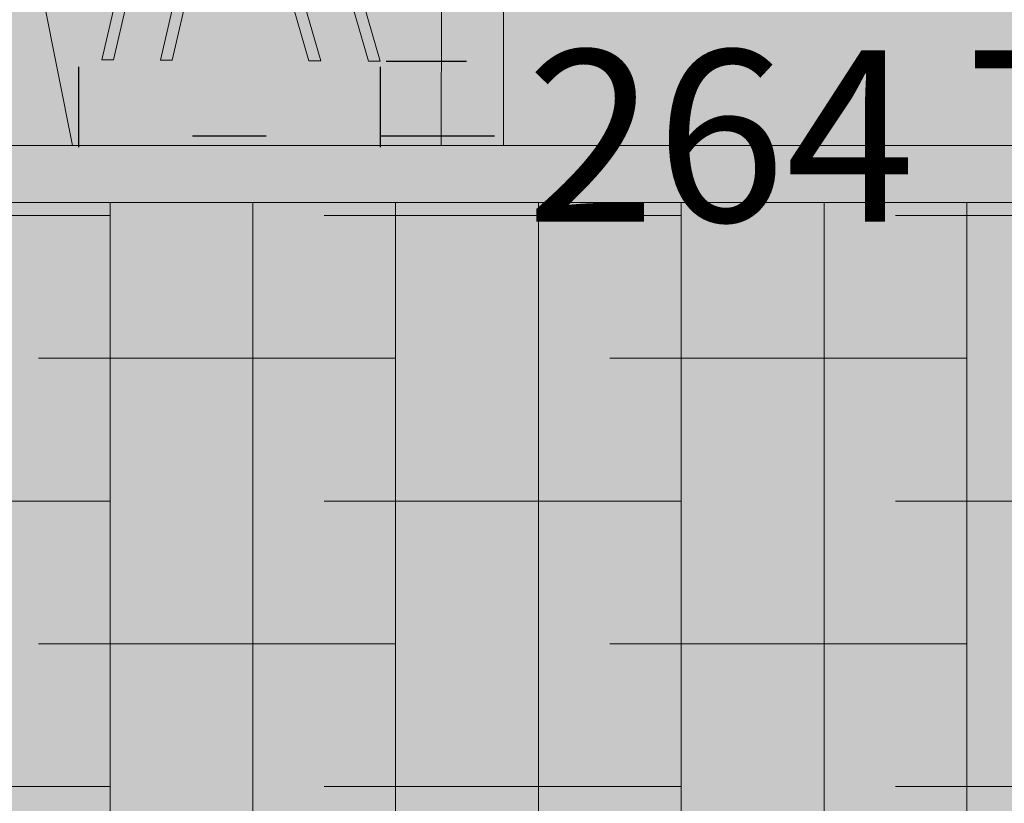
# Model space of a CAD drawing. Units: millimetres. Extents: x 11032 to 26788, y 3406 to 24505.
# Tile 4 of 78: x 15421 to 16283, y 6736 to 7421. Entities that reach past the tile are written whole.
import ezdxf

# ---------------------------------------------------------------- set-up
doc = ezdxf.new("R2010")
doc.units = ezdxf.units.MM
doc.header["$MEASUREMENT"] = 0
for name, color, linetype, lineweight in [('A-ANNO-DIMS', 2, 'Continuous', 18), ('A-FURN', 8, 'Continuous', 13), ('A-FURN-PATT', 8, 'Continuous', 13), ('A-GLAZ', 250, 'Continuous', 20), ('A-WALL-INTR', 8, 'Continuous', 18), ('A-WALL-PLIN-PATT', 253, 'Continuous', 13)]:
    doc.layers.add(name, color=color, linetype=linetype, lineweight=lineweight)
doc.layers.add('A-GLAZ-FRAM-PATT', color=250, linetype='Continuous', lineweight=13, true_color=0x262627)
doc.layers.add('A-WALL-INTR-PATT', color=251, linetype='Continuous', lineweight=13, true_color=0x6c6b6a)
doc.styles.get("Standard").update_dxf_attribs({"font": 'arial.ttf'})
doc.dimstyles.get("Standard").update_dxf_attribs({"dimtxt": 150, "dimasz": 100, "dimexe": 10, "dimexo": 5, "dimgap": 5, "dimtad": 0, "dimtih": 1, "dimtoh": 1, "dimdec": 0, "dimzin": 0, "dimdsep": 46, "dimtxsty": 'Standard', "dimcen": 0.09, "dimadec": 0, "dimazin": 0, "dimtfac": 1, "dimtdec": 0, "dimtofl": 0, "dimtmove": 0, "dimatfit": 3, "dimfxl": 1, "dimtolj": 1, "dimtzin": 0, "dimarcsym": 0})

# ---------------------------------------------------------------- blocks, each defined once
blk = doc.blocks.new('DINING-CHAIR-ELEV')
blk.add_line((228.68, 123.43), (51.04, 132.61))
for points in [[(0, 379.55), (49.45, 435.94), (114.12, 434.53)], [(61.18, 132.09), (30.79, 1.16), (20.53, 1.21), (59.55, 169.26), (0, 379.55), (61.9, 377.89)], [(111.9, 129.47), (82.06, 0.91), (71.8, 0.96), (101.76, 129.99)], [(165.28, 126.71), (201.76, 0.31), (212.19, 0.26), (175.85, 126.16)]]:
    blk.add_lwpolyline(points)
for points in [[(218.11, 123.98), (253.88, 0.05), (264.3, 0), (228.68, 123.43), (238.32, 182.18, 0.148451), (167.47, 178.33), (96.61, 174.48, 0.097012), (61.9, 377.89), (114.12, 434.53, -0.154833), (167.82, 178.46)], [(132.04, 176.4, 0.156877), (88.01, 406.21), (24.72, 407.74)]]:
    blk.add_lwpolyline(points, format="xyb")
blk = doc.blocks.new('*D16')
at = {"layer": 'A-ANNO-DIMS', "color": 0, "lineweight": -2, "transparency": 16777216}
for p, q in [((15741.74, 7821.05), (15812.13, 7821.05)), ((15802.13, 7721.05), (15802.13, 7685.69)), ((15802.13, 7485.11), (15802.13, 7520.47)), ((15741.74, 7385.11), (15812.13, 7385.11))]:
    blk.add_line(p, q, dxfattribs=at)
at = {"layer": 'A-ANNO-DIMS', "color": 0, "transparency": 16777216}
for points in [[(15785.47, 7721.05), (15818.8, 7721.05), (15802.13, 7821.05)], [(15785.47, 7485.11), (15818.8, 7485.11), (15802.13, 7385.11)]]:
    blk.add_solid(points, dxfattribs=at)
at = {"layer": 'Defpoints', "color": 0, "transparency": 16777216}
for p in [(15736.74, 7821.05), (15802.13, 7821.05), (15736.74, 7385.11)]:
    blk.add_point(p, dxfattribs=at)
at = {"layer": 'A-ANNO-DIMS', "color": 0, "transparency": 16777216, "insert": (15802.13, 7603.08), "char_height": 150, "attachment_point": 5}
blk.add_mtext('\\A1;CHAIR 436 TYP.', dxfattribs=at)
blk = doc.blocks.new('*D17')
at = {"layer": 'A-ANNO-DIMS', "color": 0, "lineweight": -2, "transparency": 16777216}
for p, q in [((15472.44, 7380.11), (15472.44, 7309.72)), ((15736.74, 7380.11), (15736.74, 7309.72)), ((15572.44, 7319.72), (15636.74, 7319.72)), ((15736.74, 7319.72), (15836.74, 7319.72))]:
    blk.add_line(p, q, dxfattribs=at)
at = {"layer": 'A-ANNO-DIMS', "color": 0, "transparency": 16777216}
for points in [[(15572.44, 7336.38), (15572.44, 7303.05), (15472.44, 7319.72)], [(15636.74, 7336.38), (15636.74, 7303.05), (15736.74, 7319.72)]]:
    blk.add_solid(points, dxfattribs=at)
at = {"layer": 'Defpoints', "color": 0, "transparency": 16777216}
for p in [(15472.44, 7385.11), (15736.74, 7385.11), (15736.74, 7319.72)]:
    blk.add_point(p, dxfattribs=at)
at = {"layer": 'A-ANNO-DIMS', "color": 0, "transparency": 16777216, "insert": (16266.37, 7319.72), "char_height": 150, "attachment_point": 5}
blk.add_mtext('\\A1;264 TYP.', dxfattribs=at)
blk = doc.blocks.new('*D36')
at = {"layer": 'A-ANNO-DIMS', "color": 0, "lineweight": -2, "transparency": 16777216}
for p, q in [((12301.26, 17115.89), (12301.26, 24416.86)), ((25397.4, 4466.4), (25397.4, 24416.86)), ((12401.26, 24406.86), (18569.2, 24406.86)), ((25297.4, 24406.86), (19129.47, 24406.86))]:
    blk.add_line(p, q, dxfattribs=at)
at = {"layer": 'A-ANNO-DIMS', "color": 0, "transparency": 16777216}
for points in [[(12401.26, 24423.52), (12401.26, 24390.19), (12301.26, 24406.86)], [(25297.4, 24423.52), (25297.4, 24390.19), (25397.4, 24406.86)]]:
    blk.add_solid(points, dxfattribs=at)
at = {"layer": 'Defpoints', "color": 0, "transparency": 16777216}
for p in [(25397.4, 24406.86), (12301.26, 17110.89), (25397.4, 4461.4)]:
    blk.add_point(p, dxfattribs=at)
at = {"layer": 'A-ANNO-DIMS', "color": 0, "transparency": 16777216, "insert": (18849.33, 24406.86), "char_height": 150, "attachment_point": 5}
blk.add_mtext('\\A1;13096', dxfattribs=at)
blk = doc.blocks.new('*D37')
at = {"layer": 'A-ANNO-DIMS', "color": 0, "lineweight": -2, "transparency": 16777216}
for p, q in [((18087.74, 23450.36), (11334.76, 23450.36)), ((11344.76, 23350.36), (11344.76, 14037.46)), ((11344.76, 4561.4), (11344.76, 13874.29)), ((12927.66, 4461.4), (11334.76, 4461.4))]:
    blk.add_line(p, q, dxfattribs=at)
at = {"layer": 'A-ANNO-DIMS', "color": 0, "transparency": 16777216}
for points in [[(11328.1, 23350.36), (11361.43, 23350.36), (11344.76, 23450.36)], [(11328.1, 4561.4), (11361.43, 4561.4), (11344.76, 4461.4)]]:
    blk.add_solid(points, dxfattribs=at)
at = {"layer": 'Defpoints', "color": 0, "transparency": 16777216}
for p in [(11344.76, 23450.36), (18092.74, 23450.36), (12932.66, 4461.4)]:
    blk.add_point(p, dxfattribs=at)
at = {"layer": 'A-ANNO-DIMS', "color": 0, "transparency": 16777216, "insert": (11344.76, 13955.88), "char_height": 150, "attachment_point": 5}
blk.add_mtext('\\A1;18989', dxfattribs=at)
blk = doc.blocks.new('*D49')
at = {"layer": 'A-ANNO-DIMS', "color": 0, "lineweight": -2, "transparency": 16777216}
for p, q in [((17953.45, 10206.41), (17953.45, 3494.9)), ((14996.4, 6406.4), (14996.4, 3494.9)), ((15096.4, 3504.9), (16244.67, 3504.9)), ((17853.45, 3504.9), (16705.18, 3504.9))]:
    blk.add_line(p, q, dxfattribs=at)
at = {"layer": 'A-ANNO-DIMS', "color": 0, "transparency": 16777216}
for points in [[(15096.4, 3521.57), (15096.4, 3488.23), (14996.4, 3504.9)], [(17853.45, 3521.57), (17853.45, 3488.23), (17953.45, 3504.9)]]:
    blk.add_solid(points, dxfattribs=at)
at = {"layer": 'Defpoints', "color": 0, "transparency": 16777216}
for p in [(17953.45, 10211.41), (14996.4, 6411.4), (17953.45, 3504.9)]:
    blk.add_point(p, dxfattribs=at)
at = {"layer": 'A-ANNO-DIMS', "color": 0, "transparency": 16777216, "insert": (16474.93, 3504.9), "char_height": 150, "attachment_point": 5}
blk.add_mtext('\\A1;2957', dxfattribs=at)
blk = doc.blocks.new('*D57')
at = {"layer": 'A-ANNO-DIMS', "color": 0, "lineweight": -2, "transparency": 16777216}
for p, q in [((14994.7, 7266.4), (14994.7, 24416.86)), ((20894.7, 7266.4), (20894.7, 24416.86)), ((15094.7, 24406.86), (17715.98, 24406.86)), ((20794.7, 24406.86), (18173.42, 24406.86))]:
    blk.add_line(p, q, dxfattribs=at)
at = {"layer": 'A-ANNO-DIMS', "color": 0, "transparency": 16777216}
for points in [[(15094.7, 24423.52), (15094.7, 24390.19), (14994.7, 24406.86)], [(20794.7, 24423.52), (20794.7, 24390.19), (20894.7, 24406.86)]]:
    blk.add_solid(points, dxfattribs=at)
at = {"layer": 'Defpoints', "color": 0, "transparency": 16777216}
for p in [(20894.7, 24406.86), (14994.7, 7261.4), (20894.7, 7261.4)]:
    blk.add_point(p, dxfattribs=at)
at = {"layer": 'A-ANNO-DIMS', "color": 0, "transparency": 16777216, "insert": (17944.7, 24406.86), "char_height": 150, "attachment_point": 5}
blk.add_mtext('\\A1;5900', dxfattribs=at)
blk = doc.blocks.new('*D60')
at = {"layer": 'A-ANNO-DIMS', "color": 0, "lineweight": -2, "transparency": 16777216}
for p, q in [((14994.7, 7266.4), (14994.7, 24416.86)), ((16344.7, 7266.4), (16344.7, 24416.86)), ((15094.7, 24406.86), (15448.04, 24406.86)), ((16244.7, 24406.86), (15891.36, 24406.86))]:
    blk.add_line(p, q, dxfattribs=at)
at = {"layer": 'A-ANNO-DIMS', "color": 0, "transparency": 16777216}
for points in [[(15094.7, 24423.52), (15094.7, 24390.19), (14994.7, 24406.86)], [(16244.7, 24423.52), (16244.7, 24390.19), (16344.7, 24406.86)]]:
    blk.add_solid(points, dxfattribs=at)
at = {"layer": 'Defpoints', "color": 0, "transparency": 16777216}
for p in [(16344.7, 24406.86), (14994.7, 7261.4), (16344.7, 7261.4)]:
    blk.add_point(p, dxfattribs=at)
at = {"layer": 'A-ANNO-DIMS', "color": 0, "transparency": 16777216, "insert": (15669.7, 24406.86), "char_height": 150, "attachment_point": 5}
blk.add_mtext('\\A1;1350', dxfattribs=at)
blk = doc.blocks.new('*D69')
at = {"layer": 'A-ANNO-DIMS', "color": 0, "lineweight": -2, "transparency": 16777216}
for p, q in [((13956.97, 9937.95), (14056.97, 9937.95)), ((14056.97, 9937.95), (15432.5, 8990.95)), ((17944.61, 7261.4), (17944.79, 7261.4)), ((17944.7, 7261.31), (17944.7, 7261.49))]:
    blk.add_line(p, q, dxfattribs=at)
at = {"layer": 'A-ANNO-DIMS', "color": 0, "transparency": 16777216}
blk.add_solid([(15441.95, 9004.68), (15423.05, 8977.22), (15514.87, 8934.24)], dxfattribs=at)
at = {"layer": 'Defpoints', "color": 0, "transparency": 16777216}
for p in [(15514.87, 8934.24), (17944.7, 7261.4)]:
    blk.add_point(p, dxfattribs=at)
at = {"layer": 'A-ANNO-DIMS', "color": 0, "transparency": 16777216, "insert": (13494.04, 9937.95), "char_height": 150, "attachment_point": 5}
blk.add_mtext('\\A1;2X R2950', dxfattribs=at)

msp = doc.modelspace()

# ---------------------------------------------------------------- hatches: boundary and pattern name
at = {"layer": 'A-FURN-PATT'}
h = msp.add_hatch(color=256, dxfattribs=at)
h.set_gradient(color1=(153, 27, 30), color2=(153, 38, 0), name='SPHERICAL')
h.paths.add_polyline_path([(15534.344, 7763), (15472.44, 7764.657), (15531.986, 7554.365), (15523.479, 7517.719), (15640.736, 7511.661), (15653.713, 7567.556, 0.0295203), (15639.906, 7563.436), (15569.055, 7559.583, 0.0970121)], flags=16)
h.paths.add_polyline_path([(15560.453, 7791.32), (15534.344, 7763, -0.0970121), (15569.055, 7559.583), (15604.48, 7561.509, 0.1568775)], flags=16)
h.paths.add_polyline_path([(15586.562, 7819.64), (15560.453, 7791.32, -0.1568775), (15604.48, 7561.509), (15640.246, 7563.454, 0.154898)], flags=17)
h.paths.add_polyline_path([(15560.453, 7791.32), (15497.165, 7792.851), (15472.44, 7764.657), (15534.344, 7763)], flags=16)
h.paths.add_polyline_path([(15586.562, 7819.64), (15521.889, 7821.046), (15497.165, 7792.851), (15560.453, 7791.32)], flags=17)
h.paths.add_polyline_path([(15790.874, 7662.689, 0.021469), (15780.879, 7659.53), (15710.028, 7655.677, 0.0970121), (15675.317, 7859.094), (15665.772, 7859.35), (15665.799, 7675.745), (15672.959, 7650.459), (15665.807, 7619.654), (15665.808, 7613.744), (15790.755, 7607.288)], flags=17)
h.paths.add_polyline_path([(15665.772, 7859.35), (15613.413, 7860.751), (15665.799, 7675.745)], flags=16)
h.paths.add_polyline_path([(15701.426, 7887.414), (15665.767, 7888.277), (15665.772, 7859.35), (15675.317, 7859.094)], flags=16)
h.paths.add_polyline_path([(15727.534, 7915.735), (15665.763, 7917.077), (15665.767, 7888.277), (15701.426, 7887.414)], flags=17)
h.paths.add_polyline_path([(15665.763, 7917.077), (15662.862, 7917.14), (15638.137, 7888.946), (15665.767, 7888.277)], flags=17)
h.paths.add_polyline_path([(15665.767, 7888.277), (15638.137, 7888.946), (15613.413, 7860.751), (15665.772, 7859.35)], flags=16)
h.paths.add_polyline_path([(15701.426, 7887.414), (15675.317, 7859.094, -0.0970121), (15710.028, 7655.677), (15745.453, 7657.604, 0.1568775)], flags=16)
h.paths.add_polyline_path([(15844.495, 7664.925), (15844.384, 7864.461), (15821.312, 7945.94), (15870.762, 8002.329), (15935.434, 8000.923, -0.1195917), (15991.005, 7804.617), (16002.667, 7804.617), (16022.264, 7889.032), (15962.718, 8099.323), (16024.622, 8097.666), (16076.839, 8154.307, -0.1548334), (16130.535, 7898.229, -0.1476694), (16201.035, 7901.954), (16191.395, 7843.208), (16202.533, 7804.617), (16299.12, 7804.617), (16297.929, 7808.825), (16347.378, 7865.214), (16412.05, 7863.808, -0.0295496), (16434.494, 7817.915), (16458.237, 7920.19), (16398.691, 8130.481), (16460.595, 8128.825), (16512.813, 8185.465, -0.1548334), (16566.508, 7929.387, -0.1476694), (16637.008, 7933.112), (16627.369, 7874.366), (16647.499, 7804.617), (16830.506, 7804.617), (16830.506, 7793.515), (16650.704, 7793.515), (16662.994, 7750.932), (16652.571, 7750.983), (16640.296, 7793.515), (16490.425, 7793.515), (16480.749, 7751.837), (16470.495, 7751.888), (16480.159, 7793.515), (16443.833, 7793.515, -0.1094051), (16465.746, 7607.731, -0.1476694), (16536.246, 7611.456), (16526.606, 7552.71), (16562.232, 7429.275), (16551.809, 7429.327), (16516.041, 7553.255), (16473.778, 7555.439), (16510.116, 7429.534), (16499.693, 7429.586), (16463.212, 7555.985), (16409.833, 7558.743), (16379.987, 7430.181), (16369.733, 7430.232), (16394.704, 7537.793), (16394.704, 7559.524), (16359.112, 7561.363), (16328.717, 7430.435), (16318.463, 7430.486), (16344.704, 7543.521), (16344.704, 7643.635), (16302.264, 7793.515), (16205.738, 7793.515), (16227.021, 7719.773), (16216.598, 7719.825), (16195.329, 7793.515), (16153.697, 7793.515), (16174.905, 7720.032), (16164.482, 7720.084), (16143.289, 7793.515), (16061.685, 7793.515), (16051.641, 7750.248, -0.0167144), (16059.629, 7748.571), (16049.99, 7689.825), (16085.615, 7566.39), (16075.192, 7566.442), (16039.424, 7690.371), (15997.161, 7692.554), (16033.5, 7566.649), (16023.077, 7566.701), (15986.595, 7693.1), (15933.216, 7695.858), (15903.371, 7567.296), (15893.116, 7567.347), (15923.072, 7696.382), (15882.495, 7698.478), (15852.409, 7568.882), (15877.716, 7481.201), (15867.293, 7481.253), (15842.372, 7567.599), (15841.846, 7567.602), (15842.08, 7568.609), (15831.524, 7605.182), (15790.755, 7607.288), (15790.744, 7602.228), (15825.6, 7481.46), (15815.177, 7481.512), (15778.696, 7607.911), (15725.317, 7610.669), (15701.389, 7507.6), (15736.743, 7385.107), (15726.32, 7385.159), (15696.749, 7487.614), (15695.471, 7482.107), (15685.217, 7482.158), (15691.06, 7507.327), (15690.552, 7509.088), (15650.881, 7511.137), (15649.743, 7506.234), (15684.627, 7385.366), (15674.204, 7385.418), (15645.103, 7486.248), (15644.2, 7482.362), (15633.946, 7482.413), (15639.413, 7505.961), (15637.723, 7511.817), (15584.344, 7514.575), (15554.498, 7386.013), (15544.244, 7386.064), (15574.2, 7515.099), (15533.623, 7517.195), (15503.228, 7386.268), (15492.974, 7386.319), (15531.986, 7554.365), (15472.44, 7764.657), (15497.165, 7792.851), (15521.889, 7821.046), (15586.562, 7819.64, -0.1548334), (15640.257, 7563.563, -0.0287549), (15653.713, 7567.556), (15665.807, 7619.654), (15665.799, 7675.745), (15613.413, 7860.751), (15638.137, 7888.946), (15662.862, 7917.14), (15665.763, 7917.077), (15727.534, 7915.735, -0.1548334), (15781.23, 7659.657, -0.1322263)])
h = msp.add_hatch(color=256, dxfattribs=at)
h.set_gradient(color1=(153, 27, 30), color2=(153, 38, 0), name='SPHERICAL')
h.paths.add_polyline_path([(15710.028, 7655.677), (15745.453, 7657.604, 0.1568775), (15701.426, 7887.414), (15675.317, 7859.094, -0.0970121)], flags=16)
h.paths.add_polyline_path([(15790.755, 7607.288), (15790.874, 7662.689, 0.021469), (15780.879, 7659.53), (15710.028, 7655.677, 0.0970121), (15675.317, 7859.094), (15665.772, 7859.35), (15665.799, 7675.745), (15672.959, 7650.459), (15665.807, 7619.654), (15665.808, 7613.744)], flags=17)
h.paths.add_polyline_path([(15653.713, 7567.556), (15665.807, 7619.654), (15665.799, 7675.745), (15613.413, 7860.751), (15662.862, 7917.14), (15727.534, 7915.735, -0.1548334), (15781.23, 7659.657, -0.1322263), (15844.495, 7664.925), (15844.384, 7864.461), (15821.312, 7945.94), (15883.216, 7944.283), (15935.434, 8000.923, -0.1195917), (15991.005, 7804.617), (16002.667, 7804.617), (16022.264, 7889.032), (15962.718, 8099.323), (16024.622, 8097.666), (16076.839, 8154.307, -0.1548334), (16130.535, 7898.229, -0.1476694), (16201.035, 7901.954), (16191.395, 7843.208), (16202.533, 7804.617), (16830.506, 7804.617), (16830.506, 7793.515), (16205.738, 7793.515), (16227.021, 7719.773), (16216.598, 7719.825), (16195.329, 7793.515), (16153.697, 7793.515), (16174.905, 7720.032), (16164.482, 7720.084), (16143.289, 7793.515), (16061.685, 7793.515), (16051.641, 7750.248, -0.0167144), (16059.629, 7748.571), (16049.99, 7689.825), (16085.615, 7566.39), (16075.192, 7566.442), (16039.424, 7690.371), (15997.161, 7692.554), (16033.5, 7566.649), (16023.077, 7566.701), (15986.595, 7693.1), (15933.216, 7695.858), (15903.371, 7567.296), (15893.116, 7567.347), (15923.072, 7696.382), (15882.495, 7698.478), (15852.409, 7568.882), (15877.716, 7481.201), (15867.293, 7481.253), (15842.372, 7567.599), (15841.846, 7567.602), (15842.08, 7568.609), (15831.524, 7605.182), (15790.755, 7607.288), (15790.744, 7602.228), (15825.6, 7481.46), (15815.177, 7481.512), (15778.696, 7607.911), (15725.317, 7610.669), (15701.389, 7507.6), (15736.743, 7385.107), (15726.32, 7385.159), (15696.749, 7487.614), (15695.471, 7482.107), (15685.217, 7482.158), (15705.262, 7568.502, 0.0841685), (15664.448, 7569.579), (15644.2, 7482.362), (15633.946, 7482.413), (15653.713, 7567.556, 0.0295203), (15639.906, 7563.436), (15569.055, 7559.583, 0.0970121), (15534.344, 7763), (15472.44, 7764.657), (15521.889, 7821.046), (15586.562, 7819.64, -0.1548334), (15640.257, 7563.563, -0.0287549)])
at = {"layer": 'A-GLAZ-FRAM-PATT'}
h = msp.add_hatch(color=256, dxfattribs=at)
h.paths.add_polyline_path([(17944.704, 7311.399), (16344.704, 7311.399), (16344.704, 7261.399), (17944.704, 7261.399)], flags=17)
h.paths.add_polyline_path([(16344.704, 7311.399), (15045.135, 7311.399, -0.9829047), (20844.273, 7311.399), (19544.704, 7311.399), (19544.704, 7261.399), (20894.704, 7261.399, 0.5148441), (16985.951, 10051.255, 0.3202679), (14994.704, 7261.399), (16344.704, 7261.399)])
h.paths.add_polyline_path([(18744.704, 7311.399), (17944.704, 7311.399), (17944.704, 7261.399), (18744.704, 7261.399)], flags=17)
h.paths.add_polyline_path([(19544.704, 7311.399), (18744.704, 7311.399), (18744.704, 7261.399), (19544.704, 7261.399)], flags=17)
h.paths.add_polyline_path([(18694.704, 7361.399), (17994.704, 7361.399), (17994.704, 7311.399), (18694.704, 7311.399)], flags=17)
h.paths.add_polyline_path([(18744.704, 7361.399), (18694.704, 7361.399), (18694.704, 7311.399), (18744.704, 7311.399)], flags=17)
h.paths.add_polyline_path([(17194.704, 7361.399), (17144.704, 7361.399), (17144.704, 7311.399), (17194.704, 7311.399)], flags=17)
h.paths.add_polyline_path([(17431.432, 7361.399), (17194.704, 7361.399), (17194.704, 7311.399), (17431.699, 7311.399)], flags=17)
h.paths.add_polyline_path([(17894.704, 7361.399), (17431.432, 7361.399), (17431.699, 7311.399), (17894.704, 7311.399)], flags=17)
h.paths.add_polyline_path([(17944.704, 7361.399), (17894.704, 7361.399), (17894.704, 7311.399), (17944.704, 7311.399)], flags=17)
h.paths.add_polyline_path([(17994.704, 7361.399), (17944.704, 7361.399), (17944.704, 7311.399), (17994.704, 7311.399)], flags=17)
at = {"layer": 'A-WALL-INTR-PATT'}
msp.add_hatch(color=256, dxfattribs=at).paths.add_polyline_path([(15447.906, 8736.527, 0.0271717), (15302.659, 8457.059), (15381.661, 7740.545), (15467.334, 7311.399), (15790.119, 7311.399), (15790.667, 7566.433), (15778.696, 7607.911), (15725.317, 7610.669), (15701.389, 7507.6), (15736.743, 7385.107), (15726.32, 7385.159), (15696.749, 7487.614), (15695.471, 7482.107), (15685.217, 7482.158), (15691.06, 7507.327), (15690.552, 7509.088), (15650.881, 7511.137), (15649.743, 7506.234), (15684.627, 7385.366), (15674.204, 7385.418), (15645.103, 7486.248), (15644.2, 7482.362), (15633.946, 7482.413), (15639.413, 7505.961), (15637.723, 7511.817), (15584.344, 7514.575), (15554.498, 7386.013), (15544.244, 7386.064), (15574.2, 7515.099), (15533.623, 7517.195), (15503.228, 7386.268), (15492.974, 7386.319), (15531.986, 7554.365), (15472.44, 7764.657)])
h = msp.add_hatch(color=256, dxfattribs=at)
h.paths.add_polyline_path([(15302.659, 8457.059, 0.0281002), (15185.248, 8153.253), (15233.282, 7717.599), (15314.374, 7311.399), (15467.334, 7311.399), (15381.661, 7740.545)])
h.paths.add_polyline_path([(16344.704, 7543.521), (16344.704, 7643.635), (16302.264, 7793.515), (16205.738, 7793.515), (16227.021, 7719.773), (16216.598, 7719.825), (16195.329, 7793.515), (16153.697, 7793.515), (16174.905, 7720.032), (16164.482, 7720.084), (16143.289, 7793.515), (16061.685, 7793.515), (16051.641, 7750.248, -0.0167144), (16059.629, 7748.571), (16049.99, 7689.825), (16085.615, 7566.39), (16075.192, 7566.442), (16039.424, 7690.371), (15997.161, 7692.554), (16033.5, 7566.649), (16023.077, 7566.701), (15986.595, 7693.1), (15933.216, 7695.858), (15903.371, 7567.296), (15893.116, 7567.347), (15923.072, 7696.382), (15882.495, 7698.478), (15852.409, 7568.882), (15877.716, 7481.201), (15867.293, 7481.253), (15844.553, 7560.041), (15844.691, 7311.399), (16344.704, 7311.399), (16344.704, 7499.3), (16328.717, 7430.435), (16318.463, 7430.486)])
h.paths.add_polyline_path([(16742.983, 7793.515), (16650.704, 7793.515), (16662.994, 7750.932), (16652.571, 7750.983), (16640.296, 7793.515), (16598.663, 7793.515), (16610.879, 7751.191), (16600.455, 7751.242), (16588.255, 7793.515), (16490.425, 7793.515), (16480.749, 7751.837), (16470.495, 7751.888), (16480.159, 7793.515), (16443.833, 7793.515, -0.1094051), (16465.746, 7607.731, -0.1476694), (16536.246, 7611.456), (16526.606, 7552.71), (16562.232, 7429.275), (16551.809, 7429.327), (16516.041, 7553.255), (16473.778, 7555.439), (16510.116, 7429.534), (16499.693, 7429.586), (16463.212, 7555.985), (16409.833, 7558.743), (16394.704, 7493.572), (16394.704, 7361.399), (16744.704, 7361.399)])
h.paths.add_polyline_path([(17094.704, 8239.696), (16741.207, 8239.696), (16742.939, 7804.617), (16768.057, 7804.617), (16785.352, 7864.542), (16775.713, 7923.288, -0.1476694), (16846.212, 7919.563, -0.1548334), (16899.908, 8175.64), (16964.58, 8177.046), (17014.03, 8120.657), (16954.484, 7910.365), (16972.017, 7834.84), (16977.75, 7834.965), (17027.199, 7778.576), (16967.653, 7568.284), (17006.665, 7400.238), (16996.411, 7400.187), (16966.016, 7531.114), (16925.439, 7529.018), (16955.395, 7399.983), (16945.141, 7399.932), (16915.295, 7528.494), (16861.916, 7525.736), (16825.435, 7399.337), (16815.012, 7399.285), (16851.35, 7525.19), (16809.087, 7523.007), (16773.319, 7399.078), (16762.896, 7399.026), (16798.521, 7522.461), (16788.882, 7581.207, -0.1476694), (16859.382, 7577.482, -0.1528132), (16911.41, 7830.579), (16902.125, 7870.575), (16848.746, 7867.817), (16830.506, 7804.617), (16830.506, 7793.515), (16827.302, 7793.515), (16812.265, 7741.418), (16801.842, 7741.366), (16816.893, 7793.515), (16775.261, 7793.515), (16760.15, 7741.159), (16749.727, 7741.107), (16764.853, 7793.515), (16742.983, 7793.515), (16744.704, 7361.399), (17094.704, 7361.399)])
h.paths.add_polyline_path([(18950.929, 7931.023), (19015.601, 7932.429), (19065.05, 7876.04), (19005.504, 7665.748), (19014.012, 7629.102, -0.129191), (19069.892, 7841.762), (19134.564, 7843.167), (19168.958, 7803.946), (19202.145, 7841.791), (19246.92, 7840.817), (19212.932, 7960.847), (19262.382, 8017.236), (19327.054, 8015.831, -0.134919), (19382.824, 7793.43), (19562.845, 7793.43, -0.1257757), (19618.686, 8000.275), (19683.358, 8001.68), (19732.808, 7945.291), (19689.807, 7793.43), (19753.644, 7793.43, -0.0966843), (19805.964, 7950.707), (19870.637, 7952.112), (19920.086, 7895.723), (19891.121, 7793.43), (20039.255, 7793.43, -0.0897865), (20089.9, 7938.993), (20154.572, 7940.399), (20204.021, 7884.01), (20144.475, 7673.718), (20152.983, 7637.072, -0.1476694), (20223.483, 7633.347, -0.1548334), (20277.178, 7889.425), (20341.85, 7890.831), (20391.3, 7834.441), (20331.754, 7624.15), (20370.766, 7456.103), (20360.512, 7456.052), (20330.117, 7586.98), (20289.54, 7584.884), (20319.496, 7455.848), (20309.241, 7455.797), (20279.396, 7584.359), (20226.017, 7581.602), (20189.536, 7455.202), (20179.112, 7455.151), (20215.451, 7581.056), (20173.188, 7578.872), (20169.478, 7566.018), (20183.488, 7505.671), (20173.234, 7505.62), (20163.789, 7546.305), (20137.42, 7454.943), (20126.997, 7454.892), (20159.149, 7566.291), (20142.839, 7636.548), (20102.261, 7634.452), (20132.217, 7505.417), (20121.963, 7505.366), (20092.117, 7633.928), (20038.738, 7631.17), (20002.257, 7504.771), (19991.834, 7504.719), (20028.172, 7630.624), (19985.91, 7628.44), (19950.141, 7504.512), (19939.718, 7504.46), (19975.344, 7627.895), (19965.704, 7686.641, -0.1476694), (20036.204, 7682.916, -0.0576487), (20037.659, 7782.328), (19887.977, 7782.328), (19860.54, 7685.431), (19899.552, 7517.385), (19889.298, 7517.334), (19858.903, 7648.261), (19818.326, 7646.165), (19848.282, 7517.13), (19838.028, 7517.079), (19808.182, 7645.641), (19754.803, 7642.883), (19718.322, 7516.484), (19707.899, 7516.432), (19744.237, 7642.337), (19701.974, 7640.154), (19698.264, 7627.3), (19712.274, 7566.953), (19702.02, 7566.902), (19692.575, 7607.587), (19666.206, 7516.225), (19655.783, 7516.173), (19687.935, 7627.573), (19671.625, 7697.83), (19631.048, 7695.733), (19661.003, 7566.698), (19650.749, 7566.647), (19620.903, 7695.209), (19567.524, 7692.451), (19531.043, 7566.052), (19520.62, 7566), (19556.959, 7691.905), (19514.696, 7689.722), (19478.928, 7565.793), (19468.505, 7565.741), (19473, 7581.318), (19466.812, 7581.349), (19431.044, 7705.278), (19388.781, 7707.461), (19425.12, 7581.556), (19414.696, 7581.608), (19378.215, 7708.007), (19324.836, 7710.765), (19318.877, 7685.094, -0.0584523), (19320.513, 7584.307, -0.1476694), (19391.013, 7588.032), (19381.373, 7529.286), (19416.999, 7405.852), (19406.576, 7405.903), (19370.808, 7529.832), (19328.545, 7532.016), (19364.883, 7406.111), (19354.46, 7406.162), (19317.979, 7532.562), (19264.6, 7535.319), (19234.754, 7406.757), (19224.5, 7406.808), (19254.456, 7535.844), (19213.879, 7537.94), (19183.484, 7407.012), (19173.23, 7407.063), (19212.242, 7575.11), (19168.16, 7730.789), (19124.467, 7576.487), (19163.48, 7408.44), (19153.225, 7408.389), (19122.83, 7539.317), (19082.253, 7537.22), (19112.209, 7408.185), (19101.955, 7408.134), (19072.109, 7536.696), (19035.898, 7534.825), (19044.517, 7497.701), (19034.262, 7497.65), (19025.754, 7534.301), (19018.73, 7533.938), (18982.249, 7407.539), (18971.826, 7407.487), (19008.164, 7533.392), (18985.177, 7532.205), (18993.246, 7497.447), (18982.992, 7497.396), (18975.033, 7531.681), (18965.902, 7531.209), (18930.133, 7407.28), (18919.71, 7407.228), (18955.336, 7530.663), (18945.696, 7589.409, -0.0318483), (18960.996, 7592.142), (18953.146, 7625.958), (18899.767, 7623.2), (18863.286, 7496.801), (18852.863, 7496.749), (18889.201, 7622.654), (18846.938, 7620.47), (18811.17, 7496.542), (18800.747, 7496.49), (18836.373, 7619.924), (18826.733, 7678.67, -0.1476694), (18897.233, 7674.946, -0.1548334)], flags=16)
h = msp.add_hatch(color=256, dxfattribs=at)
h.set_gradient(color1=(254, 234, 185), color2=(254, 204, 102), name='CURVED')
h.paths.add_polyline_path([(15260.167, 7582.928), (15062.56, 7582.722, 0.023451), (15045.135, 7311.399), (15314.374, 7311.399)])
h.paths.add_polyline_path([(15413.095, 7583.087), (15260.167, 7582.928), (15314.374, 7311.399), (15467.334, 7311.399)])
h.paths.add_polyline_path([(15531.986, 7554.365), (15523.82, 7583.203), (15413.095, 7583.087), (15467.334, 7311.399), (15790.119, 7311.399), (15790.667, 7566.433), (15785.748, 7583.476), (15718.988, 7583.406), (15701.389, 7507.6), (15736.743, 7385.107), (15726.32, 7385.159), (15696.749, 7487.614), (15695.471, 7482.107), (15685.217, 7482.158), (15691.06, 7507.327), (15690.552, 7509.088), (15650.881, 7511.137), (15649.743, 7506.234), (15684.627, 7385.366), (15674.204, 7385.418), (15646.227, 7482.352), (15633.946, 7482.413), (15639.413, 7505.961), (15637.723, 7511.817), (15584.344, 7514.575), (15554.498, 7386.013), (15544.244, 7386.064), (15574.2, 7515.099), (15533.623, 7517.195), (15503.228, 7386.268), (15492.974, 7386.319)])
h.paths.add_polyline_path([(16344.704, 7499.3), (16328.717, 7430.435), (16318.463, 7430.486), (16344.704, 7543.521), (16344.704, 7584.059), (16080.595, 7583.783), (16085.615, 7566.39), (16075.192, 7566.442), (16070.19, 7583.773), (16028.57, 7583.729), (16033.5, 7566.649), (16023.077, 7566.701), (16018.165, 7583.718), (15907.156, 7583.603), (15903.371, 7567.296), (15893.116, 7567.347), (15896.888, 7583.592), (15855.814, 7583.549), (15852.409, 7568.882), (15877.716, 7481.201), (15867.293, 7481.253), (15844.553, 7560.041), (15844.691, 7311.399), (16344.704, 7311.399)])
h.paths.add_polyline_path([(15844.553, 7560.041), (15842.372, 7567.599), (15841.846, 7567.602), (15842.08, 7568.609), (15837.773, 7583.53), (15796.153, 7583.487), (15825.6, 7481.46), (15815.177, 7481.512), (15790.667, 7566.433), (15790.119, 7311.399), (15844.691, 7311.399)])
h.paths.add_polyline_path([(16394.704, 7493.572), (16379.987, 7430.181), (16369.733, 7430.232), (16394.704, 7537.793), (16394.704, 7559.524), (16359.112, 7561.363), (16344.704, 7499.3), (16344.704, 7311.399), (17144.704, 7311.399), (17144.704, 7584.893), (17094.704, 7584.841), (17094.704, 7361.399), (16394.704, 7361.399)])
h.paths.add_polyline_path([(17430.237, 7585.191), (17194.704, 7584.945), (17194.704, 7361.399), (17431.432, 7361.399)])
h.paths.add_polyline_path([(17894.704, 7585.675), (17748.458, 7585.522), (17754.673, 7563.99), (17744.25, 7564.042), (17738.053, 7585.511), (17696.433, 7585.468), (17702.557, 7564.249), (17692.134, 7564.301), (17686.028, 7585.457), (17577.175, 7585.344), (17572.428, 7564.896), (17562.174, 7564.947), (17566.907, 7585.333), (17525.833, 7585.29), (17521.158, 7565.151), (17510.903, 7565.202), (17515.565, 7585.28), (17430.237, 7585.191), (17431.432, 7361.399), (17894.704, 7361.399)])
h.paths.add_polyline_path([(18694.704, 7586.509), (18404.857, 7586.207), (18425.604, 7496.839), (18415.35, 7496.788), (18394.593, 7586.196), (18353.54, 7586.153), (18374.333, 7496.584), (18364.079, 7496.533), (18343.276, 7586.142), (18270.386, 7586.066), (18244.373, 7495.938), (18233.95, 7495.887), (18259.974, 7586.056), (18218.329, 7586.012), (18192.257, 7495.679), (18181.834, 7495.628), (18207.918, 7586.001), (17994.704, 7585.779), (17994.704, 7361.399), (18694.704, 7361.399)])
h.paths.add_polyline_path([(19317.979, 7532.562), (19264.6, 7535.319), (19234.754, 7406.757), (19224.5, 7406.808), (19254.456, 7535.844), (19213.879, 7537.94), (19183.484, 7407.012), (19173.23, 7407.063), (19212.242, 7575.11), (19208.862, 7587.045), (19127.433, 7586.96), (19124.467, 7576.487), (19163.48, 7408.44), (19153.225, 7408.389), (19122.83, 7539.317), (19082.253, 7537.22), (19112.209, 7408.185), (19101.955, 7408.134), (19072.109, 7536.696), (19035.898, 7534.825), (19044.517, 7497.701), (19034.262, 7497.65), (19025.754, 7534.301), (19018.73, 7533.938), (18982.249, 7407.539), (18971.826, 7407.487), (19008.164, 7533.392), (18985.177, 7532.205), (18993.246, 7497.447), (18982.992, 7497.396), (18975.033, 7531.681), (18965.902, 7531.209), (18930.133, 7407.28), (18919.71, 7407.228), (18955.336, 7530.663), (18946.129, 7586.771), (18889.236, 7586.712), (18863.286, 7496.801), (18852.863, 7496.749), (18878.825, 7586.701), (18837.179, 7586.657), (18811.17, 7496.542), (18800.747, 7496.49), (18826.768, 7586.647), (18794.704, 7586.613), (18794.704, 7361.399), (19494.704, 7361.399), (19494.704, 7587.343), (19485.145, 7587.333), (19478.928, 7565.793), (19468.505, 7565.741), (19473, 7581.318), (19466.812, 7581.349), (19465.091, 7587.312), (19423.471, 7587.269), (19425.12, 7581.556), (19414.696, 7581.608), (19413.066, 7587.258), (19390.882, 7587.235), (19381.373, 7529.286), (19416.999, 7405.852), (19406.576, 7405.903), (19370.808, 7529.832), (19328.545, 7532.016), (19364.883, 7406.111), (19354.46, 7406.162)])
h.paths.add_polyline_path([(19990.261, 7587.86), (19974.192, 7587.843), (19950.141, 7504.512), (19939.718, 7504.46), (19963.781, 7587.832), (19883.217, 7587.748), (19899.552, 7517.385), (19889.298, 7517.334), (19872.954, 7587.737), (19831.9, 7587.695), (19848.282, 7517.13), (19838.028, 7517.079), (19821.637, 7587.684), (19738.846, 7587.598), (19718.322, 7516.484), (19707.899, 7516.432), (19728.435, 7587.587), (19707.489, 7587.565), (19712.274, 7566.953), (19702.02, 7566.902), (19697.225, 7587.554), (19686.79, 7587.543), (19666.206, 7516.225), (19655.783, 7516.173), (19676.379, 7587.532), (19656.172, 7587.511), (19661.003, 7566.698), (19650.749, 7566.647), (19645.908, 7587.501), (19544.704, 7587.395), (19544.704, 7311.399), (19990.261, 7311.399)])
h.paths.add_polyline_path([(20190.261, 7455.206), (20179.112, 7455.151), (20190.261, 7493.779), (20190.261, 7579.754), (20173.188, 7578.872), (20169.478, 7566.018), (20183.488, 7505.671), (20173.234, 7505.62), (20163.789, 7546.305), (20137.42, 7454.943), (20126.997, 7454.892), (20159.149, 7566.291), (20154.102, 7588.03), (20113.048, 7587.988), (20132.217, 7505.417), (20121.963, 7505.366), (20102.785, 7587.977), (20026.249, 7587.897), (20002.257, 7504.771), (19990.261, 7504.711), (19990.261, 7311.399), (20190.261, 7311.399)])
h.paths.add_polyline_path([(20340.261, 7543.283), (20330.117, 7586.98), (20289.54, 7584.884), (20319.496, 7455.848), (20309.241, 7455.797), (20279.396, 7584.359), (20226.017, 7581.602), (20190.261, 7457.717), (20190.261, 7311.399), (20340.261, 7311.399)])
h.paths.add_polyline_path([(20826.171, 7588.731), (20340.261, 7588.225), (20340.261, 7587.504), (20370.766, 7456.103), (20360.512, 7456.052), (20340.261, 7543.283), (20340.261, 7311.399), (20844.273, 7311.399, 0.0239726)])
at = {"layer": 'A-WALL-PLIN-PATT'}
h = msp.add_hatch(color=256, dxfattribs=at)
h.set_gradient(color1=(99, 100, 102), color2=(199, 200, 202), name='CYLINDER')
edge = h.paths.add_edge_path()
edge.add_arc((17944.704, 7261.399), 2950, 180, 181.942602)
edge.add_line((14996.399, 7161.399), (12932.665, 7161.399))
edge.add_line((12932.665, 7161.399), (12932.665, 6411.399))
edge.add_line((12932.665, 6411.399), (25397.404, 6411.399))
edge.add_line((25397.404, 6411.399), (25397.404, 7161.399))
edge.add_line((25397.404, 7161.399), (22955.171, 7161.399))
edge.add_spline(control_points=[(22955.171, 7161.399), (22875.95, 7159.113), (22796.729, 7156.828), (22718.347, 7161.399)], knot_values=[0, 0, 0, 0, 236.623895, 236.623895, 236.623895, 236.623895], degree=3, periodic=0)
edge.add_spline(control_points=[(22718.347, 7161.399), (22709.27, 7161.929), (22517.84, 7175.049), (22332.009, 7233.921), (22155.123, 7291.176)], knot_values=[236.623895, 236.623895, 236.623895, 236.623895, 264.0278501, 815.2441458, 815.2441458, 815.2441458, 815.2441458], degree=3, periodic=0)
edge.add_line((22155.123, 7291.176), (22155.123, 7161.399))
edge.add_line((22155.123, 7161.399), (20893.008, 7161.399))
edge.add_arc((17944.704, 7261.399), 2950, 358.057398, 360)
edge.add_line((20894.704, 7261.399), (14994.704, 7261.399))
h.paths.add_polyline_path([(14996.399, 6261.399), (14822.389, 6162.807), (21067.019, 6162.807), (20893.008, 6261.399)])
h.paths.add_polyline_path([(14822.224, 6012.807), (14648.718, 5913.331), (21240.69, 5913.331), (21067.183, 6012.807)])
h.paths.add_polyline_path([(21414.634, 5661.399), (21414.635, 5662.395), (21241.977, 5763.336), (14647.43, 5763.336), (14474.772, 5662.395), (14474.774, 5661.399)])
h.paths.add_polyline_path([(14474.964, 5512.395), (14302.433, 5411.236), (21586.974, 5411.236), (21414.443, 5512.395)])
h.paths.add_polyline_path([(14301.435, 5261.24), (14128.313, 5161.097), (21761.094, 5161.097), (21587.972, 5261.24)])
h.paths.add_polyline_path([(22722.526, 4461.399), (21760.979, 5011.097), (14128.428, 5011.097), (13166.882, 4461.399)])
h = msp.add_hatch(dxfattribs=at)
h.set_pattern_fill('ANSI38', color=256, scale=1000, angle=45, style=0)
edge = h.paths.add_edge_path()
edge.add_line((25397.404, 6411.399), (25397.404, 7161.399))
edge.add_line((25397.404, 7161.399), (22955.171, 7161.399))
edge.add_spline(control_points=[(22955.171, 7161.399), (22875.95, 7159.113), (22796.729, 7156.828), (22718.347, 7161.399)], knot_values=[0, 0, 0, 0, 236.623895, 236.623895, 236.623895, 236.623895], degree=3, periodic=0)
edge.add_spline(control_points=[(22718.347, 7161.399), (22709.27, 7161.929), (22517.84, 7175.049), (22332.009, 7233.921), (22155.123, 7291.176)], knot_values=[236.623895, 236.623895, 236.623895, 236.623895, 264.0278501, 815.2441458, 815.2441458, 815.2441458, 815.2441458], degree=3, periodic=0)
edge.add_line((22155.123, 7291.176), (22155.123, 7161.399))
edge.add_line((22155.123, 7161.399), (20893.008, 7161.399))
edge.add_arc((17944.704, 7261.399), 2950, 358.057398, 360)
edge.add_line((20894.704, 7261.399), (14994.704, 7261.399))
edge.add_arc((17944.704, 7261.399), 2950, 180, 181.942602)
edge.add_line((14996.399, 7161.399), (12932.665, 7161.399))
edge.add_line((12932.665, 7161.399), (12932.665, 6411.399))
edge.add_line((12932.665, 6411.399), (25397.404, 6411.399))

# ---------------------------------------------------------------- linework, layer by layer
at = {"layer": 'A-GLAZ'}
for p, q in [((15045.135, 7311.399), (20844.273, 7311.399)), ((14994.704, 7261.399), (20894.704, 7261.399))]:
    msp.add_line(p, q, dxfattribs=at)
for radius, start, end in [(2900, 0.987907, 179.012093), (2950, 108.965621, 181.942602)]:
    msp.add_arc((17944.704, 7261.399), radius, start, end, dxfattribs=at)
at = {"layer": 'A-WALL-INTR'}
for p, q in [((15843.607, 9260.247), (15844.691, 7311.399)), ((15790.119, 7311.399), (15794.195, 9206.987)), ((15467.334, 7311.399), (15381.661, 7740.545))]:
    msp.add_line(p, q, dxfattribs=at)

# ---------------------------------------------------------------- block references
at = {"layer": 'A-FURN'}
msp.add_blockref('DINING-CHAIR-ELEV', (15472.44, 7385.107), dxfattribs=at)

# ---------------------------------------------------------------- dimensions: what is measured, and where the dimension line sits
at = {"layer": 'A-ANNO-DIMS'}
for base, p1, p2, picture, middle in [((25397.404, 24406.858), (12301.265, 17110.885), (25397.404, 4461.399), '*D36', (18849.334, 24406.858)), ((20894.704, 24406.858), (14994.704, 7261.399), (20894.704, 7261.399), '*D57', (17944.704, 24406.858)), ((16344.704, 24406.858), (14994.704, 7261.399), (16344.704, 7261.399), '*D60', (15669.704, 24406.858)), ((17953.455, 3504.899), (14996.399, 6411.399), (17953.455, 10211.41), '*D49', (16474.927, 3504.899))]:
    dim = msp.add_linear_dim(base=base, p1=p1, p2=p2, dimstyle='Standard', override={"dimdec": 0, "dimlfac": 1, "dimrnd": 0, "dimzin": 0, "dimdsep": 46, "dimlunit": 2}, dxfattribs=at)
    dim.commit()
    dim.dimension.update_dxf_attribs({"geometry": picture, "text_midpoint": middle})
dim = msp.add_linear_dim(base=(11344.765, 23450.358), p1=(12932.665, 4461.399), p2=(18092.739, 23450.358), angle=90, dimstyle='Standard', override={"dimdec": 0, "dimlfac": 1, "dimrnd": 0, "dimzin": 0, "dimdsep": 46, "dimlunit": 2}, dxfattribs=at)
dim.commit()
dim.dimension.update_dxf_attribs({"geometry": '*D37', "text_midpoint": (11344.765, 13955.879)})
dim = msp.add_radius_dim(center=(17944.704, 7261.399), mpoint=(15514.87, 8934.244), text='2X <>', dimstyle='Standard', override={"dimdec": 0, "dimlfac": 1, "dimrnd": 0, "dimzin": 0, "dimdsep": 46, "dimlunit": 2}, dxfattribs=at)
dim.commit()
dim.dimension.update_dxf_attribs({"geometry": '*D69', "text_midpoint": (13494.04, 9937.951), "dimtype": 164})
dim = msp.add_linear_dim(base=(15802.134, 7821.046), p1=(15736.743, 7385.107), p2=(15736.743, 7821.046), angle=90, text='CHAIR <> TYP.', dimstyle='Standard', override={"dimdec": 0, "dimlfac": 1, "dimrnd": 0, "dimzin": 0, "dimdsep": 46, "dimlunit": 2}, dxfattribs=at)
dim.commit()
dim.dimension.update_dxf_attribs({"geometry": '*D16', "text_midpoint": (15802.134, 7603.076)})
dim = msp.add_linear_dim(base=(15736.743, 7319.716), p1=(15472.44, 7385.107), p2=(15736.743, 7385.107), text='<> TYP.', dimstyle='Standard', override={"dimdec": 0, "dimlfac": 1, "dimrnd": 0, "dimzin": 0, "dimdsep": 46, "dimlunit": 2}, dxfattribs=at)
dim.commit()
dim.dimension.update_dxf_attribs({"geometry": '*D17', "text_midpoint": (16266.368, 7319.716)})

doc.saveas('drawing.dxf')
